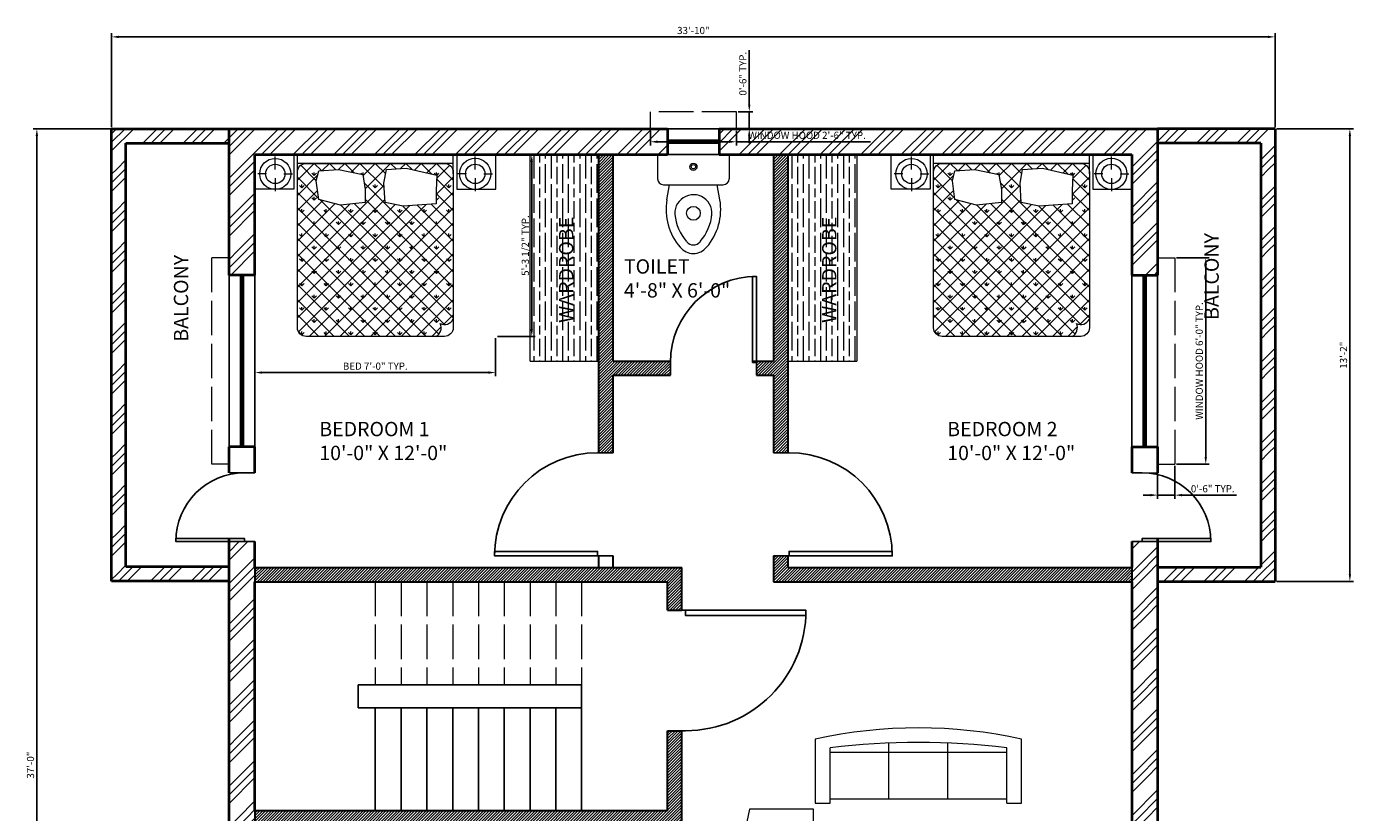
# Model space of a CAD drawing. Units: inches. Extents: x 2443635 to 2446153, y 1826255 to 1827341.
# Tile 10 of 16: x 2444253 to 2444716, y 1827067 to 1827341. Entities that reach past the tile are written whole.
import ezdxf

# ---------------------------------------------------------------- set-up
doc = ezdxf.new("R2010")
doc.units = ezdxf.units.IN
doc.linetypes.add('ACAD_ISO02W100', pattern=[15, 12, -3])
for name, color, linetype, lineweight in [('A-DIMS', 1, 'Continuous', 18), ('A-DOOR', 2, 'Continuous', 25), ('A-DOOR-HIDN', 2, 'ACAD_ISO02W100', 18), ('A-FLOR-CASE', 8, 'Continuous', 18), ('A-FLOR-CASE-PATT', 252, 'Continuous', 13), ('A-FLOR-FIXT', 9, 'Continuous', 18), ('A-FURN', 6, 'Continuous', 18), ('A-ROOM', 4, 'Continuous', 18), ('A-STAIR', 7, 'Continuous', 25), ('A-STAIR-OVHD', 7, 'ACAD_ISO02W100', 18), ('A-WALL-EXT', 7, 'Continuous', 40), ('A-WALL-INT', 9, 'Continuous', 30), ('A-WALL-OVHD', 7, 'ACAD_ISO02W100', 18), ('A-WALL-PATT', 8, 'Continuous', 13), ('A-WINDOW', 4, 'Continuous', 25)]:
    doc.layers.add(name, color=color, linetype=linetype, lineweight=lineweight)
doc.styles.get("Standard").update_dxf_attribs({"font": 'arial.ttf'})
doc.dimstyles.new('ISO-25', dxfattribs={"dimtxt": 2.5, "dimasz": 2.5, "dimexe": 1.25, "dimexo": 0.625, "dimtad": 1, "dimlunit": 4, "dimtxsty": 'Standard', "dimcen": 2.5, "dimadec": 0, "dimazin": 0, "dimtfac": 1, "dimtmove": 0, "dimatfit": 3, "dimfxl": 1, "dimarcsym": 0})

# ---------------------------------------------------------------- blocks, each defined once
blk = doc.blocks.new('*X6')
at = {"color": 0}
for p, q in [((0, 0), (0, 0)), ((-707, -141), (-734, -115)), ((-707, -141), (-707, -104)), ((-707, -141), (-681, -115)), ((-566, 0), (-566, 0)), ((-566, 0), (-566, 0)), ((-283, 0), (-283, 0)), ((-283, 0), (-283, 0)), ((-156, -126), (-168, -115)), ((-141, -141), (-142, -140)), ((-141, -141), (-141, -104)), ((-141, -141), (-115, -115)), ((120, -120), (115, -115)), ((283, 0), (283, 0)), ((566, 0), (566, 0)), ((699, -134), (681, -115)), ((707, -135), (707, -104)), ((710, -139), (734, -115)), ((-849, -283), (-875, -256)), ((-849, -283), (-849, -245)), ((-849, -283), (-822, -256)), ((0, -283), (-27, -256)), ((0, -283), (0, -245)), ((0, -283), (27, -256)), ((849, -283), (822, -256)), ((849, -283), (849, -245)), ((849, -283), (875, -256)), ((-707, -424), (-734, -398)), ((-707, -424), (-707, -387)), ((-707, -424), (-681, -398)), ((-116, -399), (-115, -398)), ((707, -424), (703, -420)), ((707, -424), (707, -387)), ((707, -424), (734, -398)), ((-849, -566), (-875, -539)), ((-849, -566), (-849, -528)), ((-849, -566), (-822, -539)), ((-566, -566), (-592, -539)), ((-566, -566), (-566, -528)), ((-566, -566), (-539, -539)), ((-283, -566), (-309, -539)), ((-283, -566), (-283, -528)), ((-283, -566), (-256, -539)), ((0, -566), (-27, -539)), ((0, -566), (0, -528)), ((0, -566), (27, -539)), ((283, -566), (256, -539)), ((283, -566), (283, -528)), ((283, -566), (309, -539)), ((566, -566), (539, -539)), ((566, -566), (566, -528)), ((566, -566), (592, -539)), ((849, -566), (822, -539)), ((849, -566), (849, -528)), ((849, -566), (875, -539)), ((-707, -707), (-734, -681)), ((-707, -707), (-707, -670)), ((-707, -707), (-681, -681)), ((-424, -707), (-451, -681)), ((-424, -707), (-424, -670)), ((-424, -707), (-398, -681)), ((-141, -707), (-168, -681)), ((-141, -707), (-141, -670)), ((-141, -707), (-115, -681)), ((141, -707), (115, -681)), ((141, -707), (141, -670)), ((141, -707), (168, -681)), ((424, -707), (398, -681)), ((424, -707), (424, -670)), ((424, -707), (451, -681)), ((707, -707), (681, -681)), ((707, -707), (707, -670)), ((707, -707), (734, -681)), ((-849, -849), (-875, -822)), ((-849, -849), (-849, -811)), ((-849, -849), (-822, -822)), ((-566, -849), (-592, -822)), ((-566, -849), (-566, -811)), ((-566, -849), (-539, -822)), ((-283, -849), (-309, -822)), ((-283, -849), (-283, -811)), ((-283, -849), (-256, -822)), ((0, -849), (-27, -822)), ((0, -849), (0, -811)), ((0, -849), (27, -822)), ((283, -849), (256, -822)), ((283, -849), (283, -811)), ((283, -849), (309, -822)), ((566, -849), (539, -822)), ((566, -849), (566, -811)), ((566, -849), (592, -822)), ((849, -849), (822, -822)), ((849, -849), (849, -811)), ((849, -849), (875, -822)), ((-707, -990), (-734, -963)), ((-707, -990), (-707, -952)), ((-707, -990), (-681, -963)), ((-424, -990), (-451, -963)), ((-424, -990), (-424, -952)), ((-424, -990), (-398, -963)), ((-141, -990), (-168, -963)), ((-141, -990), (-141, -952)), ((-141, -990), (-115, -963)), ((141, -990), (115, -963)), ((141, -990), (141, -952)), ((141, -990), (168, -963)), ((424, -990), (398, -963)), ((424, -990), (424, -952)), ((424, -990), (451, -963)), ((707, -990), (681, -963)), ((707, -990), (707, -952)), ((707, -990), (734, -963)), ((-849, -1131), (-875, -1105)), ((-849, -1131), (-849, -1094)), ((-849, -1131), (-822, -1105)), ((-566, -1131), (-592, -1105)), ((-566, -1131), (-566, -1094)), ((-566, -1131), (-539, -1105)), ((-283, -1131), (-309, -1105)), ((-283, -1131), (-283, -1094)), ((-283, -1131), (-256, -1105)), ((0, -1131), (-27, -1105)), ((0, -1131), (0, -1094)), ((0, -1131), (27, -1105)), ((283, -1131), (256, -1105)), ((283, -1131), (283, -1094)), ((283, -1131), (309, -1105)), ((566, -1131), (539, -1105)), ((566, -1131), (566, -1094)), ((566, -1131), (592, -1105)), ((849, -1131), (822, -1105)), ((849, -1131), (849, -1094)), ((849, -1131), (875, -1105)), ((-849, -1414), (-849, -1377)), ((-707, -1273), (-734, -1246)), ((-707, -1273), (-707, -1235)), ((-707, -1273), (-681, -1246)), ((-566, -1414), (-566, -1377)), ((-424, -1273), (-451, -1246)), ((-424, -1273), (-424, -1235)), ((-424, -1273), (-398, -1246)), ((-283, -1414), (-283, -1377)), ((-141, -1273), (-168, -1246)), ((-141, -1273), (-141, -1235)), ((-141, -1273), (-115, -1246)), ((0, -1414), (0, -1377)), ((141, -1273), (115, -1246)), ((141, -1273), (141, -1235)), ((141, -1273), (168, -1246)), ((283, -1414), (283, -1377)), ((424, -1273), (398, -1246)), ((424, -1273), (424, -1235)), ((424, -1273), (451, -1246)), ((566, -1414), (566, -1377)), ((707, -1273), (681, -1246)), ((707, -1273), (707, -1235)), ((707, -1273), (734, -1246)), ((849, -1414), (849, -1377)), ((-849, -1414), (-875, -1388)), ((-849, -1414), (-822, -1388)), ((-707, -1556), (-734, -1529)), ((-707, -1556), (-707, -1518)), ((-707, -1556), (-681, -1529)), ((-566, -1414), (-592, -1388)), ((-566, -1414), (-539, -1388)), ((-424, -1556), (-451, -1529)), ((-424, -1556), (-424, -1518)), ((-424, -1556), (-398, -1529)), ((-283, -1414), (-309, -1388)), ((-283, -1414), (-256, -1388)), ((-141, -1556), (-168, -1529)), ((-141, -1556), (-141, -1518)), ((-141, -1556), (-115, -1529)), ((0, -1414), (-27, -1388)), ((0, -1414), (27, -1388)), ((141, -1556), (115, -1529)), ((141, -1556), (141, -1518)), ((141, -1556), (168, -1529)), ((283, -1414), (256, -1388)), ((283, -1414), (309, -1388)), ((424, -1556), (398, -1529)), ((424, -1556), (424, -1518)), ((424, -1556), (451, -1529)), ((566, -1414), (539, -1388)), ((566, -1414), (592, -1388)), ((707, -1556), (681, -1529)), ((707, -1556), (707, -1518)), ((707, -1556), (734, -1529)), ((849, -1414), (822, -1388)), ((849, -1414), (875, -1388)), ((-849, -1697), (-875, -1671)), ((-849, -1697), (-849, -1660)), ((-849, -1697), (-822, -1671)), ((-566, -1697), (-592, -1671)), ((-566, -1697), (-566, -1660)), ((-566, -1697), (-539, -1671)), ((-283, -1697), (-309, -1671)), ((-283, -1697), (-283, -1660)), ((-283, -1697), (-256, -1671)), ((0, -1697), (-27, -1671)), ((0, -1697), (0, -1660)), ((0, -1697), (27, -1671)), ((283, -1697), (256, -1671)), ((283, -1697), (283, -1660)), ((283, -1697), (309, -1671)), ((566, -1697), (539, -1671)), ((566, -1697), (566, -1660)), ((566, -1697), (592, -1671)), ((849, -1697), (822, -1671)), ((849, -1697), (849, -1660)), ((849, -1697), (875, -1671)), ((-707, -1838), (-734, -1812)), ((-707, -1838), (-707, -1801)), ((-707, -1838), (-681, -1812)), ((-424, -1838), (-451, -1812)), ((-424, -1838), (-424, -1801)), ((-424, -1838), (-398, -1812)), ((-141, -1838), (-168, -1812)), ((-141, -1838), (-141, -1801)), ((-141, -1838), (-115, -1812)), ((141, -1838), (115, -1812)), ((141, -1838), (141, -1801)), ((141, -1838), (168, -1812)), ((424, -1838), (398, -1812)), ((424, -1838), (424, -1801)), ((424, -1838), (451, -1812)), ((707, -1838), (681, -1812)), ((707, -1838), (707, -1801)), ((707, -1838), (734, -1812)), ((-849, -1980), (-875, -1953)), ((-849, -1980), (-849, -1942)), ((-849, -1980), (-822, -1953)), ((-566, -1980), (-592, -1953)), ((-566, -1980), (-566, -1942)), ((-566, -1980), (-539, -1953)), ((-283, -1980), (-309, -1953)), ((-283, -1980), (-283, -1942)), ((-283, -1980), (-256, -1953)), ((0, -1980), (-27, -1953)), ((0, -1980), (0, -1942)), ((0, -1980), (27, -1953)), ((283, -1980), (256, -1953)), ((283, -1980), (283, -1942)), ((283, -1980), (309, -1953)), ((566, -1980), (539, -1953)), ((566, -1980), (566, -1942)), ((566, -1980), (592, -1953))]:
    blk.add_line(p, q, dxfattribs=at)
blk = doc.blocks.new('*X5')
at = {"color": 0}
for p, q in [((-900, -193), (-707, 0)), ((-623, -84), (-707, 0)), ((-614, -83), (-530, 0)), ((-457, -74), (-530, 0)), ((-425, -72), (-354, 0)), ((-245, -108), (-354, 0)), ((-278, -101), (-177, 0)), ((103, -280), (-177, 0)), ((-142, -142), (0, 0)), ((-117, -294), (177, 0)), ((120, -120), (0, 0)), ((241, -64), (177, 0)), ((292, -61), (354, 0)), ((426, -72), (354, 0)), ((452, -78), (530, 0)), ((654, -123), (530, 0)), ((596, -111), (707, 0)), ((900, -193), (707, 0)), ((-900, -370), (-667, -137)), ((-683, -201), (-862, -22)), ((708, -175), (862, -22)), ((-656, -405), (-900, -161)), ((-900, -1254), (101, -252)), ((900, -1254), (-128, -225)), ((703, -358), (900, -161)), ((900, -370), (708, -178)), ((-900, -546), (-668, -314)), ((735, -1973), (-900, -337)), ((-900, -1430), (112, -418)), ((-900, -723), (-605, -429)), ((-763, -2000), (900, -337)), ((801, -1862), (-641, -419)), ((900, -1430), (-116, -415)), ((900, -546), (703, -349)), ((-900, -900), (-465, -465)), ((-900, -1077), (-293, -470)), ((-900, -1607), (231, -476)), ((-900, -1784), (394, -489)), ((586, -2000), (-900, -514)), ((-888, -1948), (586, -475)), ((-586, -2000), (900, -514)), ((900, -1784), (-404, -480)), ((900, -1607), (-243, -465)), ((900, -1077), (317, -494)), ((900, -900), (483, -483)), ((900, -723), (647, -470)), ((409, -2000), (-900, -691)), ((-409, -2000), (900, -691)), ((232, -2000), (-900, -868)), ((-232, -2000), (900, -868)), ((55, -2000), (-900, -1045)), ((-55, -2000), (900, -1045)), ((-121, -2000), (-900, -1221)), ((121, -2000), (900, -1221)), ((-298, -2000), (-900, -1398)), ((298, -2000), (900, -1398)), ((-475, -2000), (-900, -1575)), ((475, -2000), (900, -1575)), ((-652, -2000), (-900, -1752)), ((790, -1861), (900, -1752)), ((-835, -1994), (-894, -1935)), ((652, -2000), (761, -1890))]:
    blk.add_line(p, q, dxfattribs=at)
blk = doc.blocks.new('A$C190D2546')
at = {"layer": 'A-FURN'}
for p, q in [((285, 1928), (285, 2078)), ((541, 2100), (2341, 2100)), ((541, 1881), (541, 2100)), ((2341, 2000), (541, 2000)), ((2341, 1881), (2341, 2100)), ((2596, 1929), (2596, 2079)), ((185, 1878), (85, 1878)), ((385, 1878), (485, 1878)), ((2496, 1879), (2396, 1879)), ((2696, 1879), (2796, 1879)), ((285, 1828), (285, 1678)), ((2596, 1829), (2596, 1679))]:
    blk.add_line(p, q, dxfattribs=at)
for points in [[(500, 2101), (500, 1701), (50, 1701), (50, 2101)], [(2382, 2101), (2382, 1701), (2832, 1701), (2832, 2101)], [(787, 1584), (758, 1799), (787, 1914), (1016, 1928), (1296, 1871), (1325, 1699), (1325, 1548), (1038, 1519)], [(1555, 1548), (1541, 1771), (1569, 1928), (1799, 1943), (2151, 1864), (2144, 1685), (2144, 1534), (1763, 1505)]]:
    blk.add_lwpolyline(points, close=True, dxfattribs=at)
blk.add_lwpolyline([(641, 2000), (2241, 2000, -0.414214), (2341, 1900), (2341, 100, -0.414214), (2241, 0), (641, 0, -0.414214), (541, 100), (541, 1900, -0.414214)], format="xyb", close=True, dxfattribs=at)
for centre, radius in [((285, 1878), 180), ((2596, 1879), 180), ((285, 1878), 112), ((2596, 1879), 112)]:
    blk.add_circle(centre, radius, dxfattribs=at)
for centre, start, end in [((2241, 250), 243.4349, 333.4349), ((2091, 100), 296.5651, 26.5651)]:
    blk.add_arc(centre, 112, start, end, dxfattribs=at)
for name in ['*X5', '*X6']:
    blk.add_blockref(name, (1441, 2000), dxfattribs=at)
blk = doc.blocks.new('*U2')
for p, q in [((0, 0), (0, -6)), ((40, 0), (40, -6))]:
    blk.add_line(p, q)
blk.add_lwpolyline([(0, 0), (0, 40), (1.75, 40), (1.75, 0)], close=True)
blk.add_arc((0, 0), 40, 0, 90)
blk = doc.blocks.new('*U3')
for p, q in [((0, 0), (0, -6)), ((-40, 0), (-40, -6))]:
    blk.add_line(p, q)
blk.add_lwpolyline([(0, 0), (0, 40), (-1.75, 40), (-1.75, 0)], close=True)
blk.add_arc((0, 0), 40, 90, 180)
blk = doc.blocks.new('*U14')
for p, q in [((0, 0), (0, -6)), ((40, 0), (40, -6))]:
    blk.add_line(p, q)
blk.add_lwpolyline([(0, 0), (0, 40), (1.75, 40), (1.75, 0)], close=True)
blk.add_arc((0, 0), 40, 0, 90)
blk = doc.blocks.new('SOFA-3-SEAT')
at = {"transparency": 33554687}
for p, q in [((0, 22.29), (0, 0)), ((5.14, 0), (5.14, 19.31)), ((25.71, 1.34), (25.71, 20.94)), ((46.29, 1.34), (46.29, 20.94)), ((66.86, 0), (66.86, 19.31)), ((72, 0), (72, 22.29)), ((66.86, 17.67), (5.14, 17.67)), ((0, 0), (5.14, 0)), ((66.86, 1.34), (5.14, 1.34)), ((66.86, 0), (72, 0))]:
    blk.add_line(p, q, dxfattribs=at)
for centre, radius, start, end in [((36, -137.71), 164, 77.3196, 102.6804), ((36, -239.71), 260.86, 83.2065, 96.7935)]:
    blk.add_arc(centre, radius, start, end, dxfattribs=at)
blk = doc.blocks.new('WIN-18-PLAN')
at = {"transparency": 33554687}
for p, q in [((18, 9), (0, 9)), ((0, 9), (0, 0)), ((0, 5), (18, 5)), ((0.5, 5), (0.5, 4)), ((17.5, 4), (17.5, 5)), ((18, 0), (18, 9)), ((0, 4), (18, 4)), ((0.5, 4.5), (18, 4.5)), ((0, 0), (18, 0))]:
    blk.add_line(p, q, dxfattribs=at)
blk = doc.blocks.new('WIN-60-PLAN')
at = {"transparency": 33554687}
for p, q in [((0, 0), (0, 60)), ((0, 60), (9, 60)), ((4, 60), (4, 0)), ((4, 59.5), (5, 59.5)), ((4.5, 59.5), (4.5, 0.5)), ((5, 60), (5, 0)), ((9, 60), (9, 0)), ((5, 0.5), (4, 0.5)), ((9, 0), (0, 0))]:
    blk.add_line(p, q, dxfattribs=at)
blk = doc.blocks.new('WIN-60-STRIP-PLAN')
at = {"transparency": 33554687}
for p, q in [((0, 0), (0, 60)), ((4, 60), (4, 0)), ((4.5, 59.5), (4.5, 0.5)), ((5, 60), (5, 0)), ((9, 60), (9, 0))]:
    blk.add_line(p, q, dxfattribs=at)
blk = doc.blocks.new('WINDOW-HOOD-72-PLAN')
at = {"transparency": 33554687}
for p, q in [((0, 72), (6, 72)), ((6, 72), (6, 0)), ((0, 0), (6, 0))]:
    blk.add_line(p, q, dxfattribs=at)
blk = doc.blocks.new('WINDOW-HOOD-30-PLAN')
at = {"transparency": 33554687}
for p, q in [((30, 6), (0, 6)), ((0, 0), (0, 6)), ((30, 0), (30, 6))]:
    blk.add_line(p, q, dxfattribs=at)
blk = doc.blocks.new('*D52')
at = {"layer": 'A-DIMS', "color": 0, "lineweight": -2, "transparency": 16777216}
for p, q in [((2444332.55, 1827232.23), (2444332.55, 1827219)), ((2444416.55, 1827232.23), (2444416.55, 1827219)), ((2444335.05, 1827220.25), (2444414.05, 1827220.25))]:
    blk.add_line(p, q, dxfattribs=at)
at = {"layer": 'A-DIMS', "color": 0, "transparency": 16777216}
for points in [[(2444335.05, 1827220.67), (2444335.05, 1827219.84), (2444332.55, 1827220.25)], [(2444414.05, 1827220.67), (2444414.05, 1827219.84), (2444416.55, 1827220.25)]]:
    blk.add_solid(points, dxfattribs=at)
at = {"layer": 'Defpoints', "color": 0, "transparency": 16777216}
for p in [(2444332.55, 1827232.85), (2444416.55, 1827232.85), (2444416.55, 1827220.25)]:
    blk.add_point(p, dxfattribs=at)
at = {"layer": 'A-DIMS', "color": 0, "transparency": 16777216, "insert": (2444374.55, 1827222.16), "char_height": 2.5, "attachment_point": 5}
blk.add_mtext('BED 7\'-0" TYP.', dxfattribs=at)
blk = doc.blocks.new('*D53')
at = {"layer": 'A-DIMS', "color": 0, "lineweight": -2, "transparency": 16777216}
for p, q in [((2444417.18, 1827296.29), (2444430.4, 1827296.29)), ((2444429.15, 1827235.35), (2444429.15, 1827293.79)), ((2444417.18, 1827232.85), (2444430.4, 1827232.85))]:
    blk.add_line(p, q, dxfattribs=at)
at = {"layer": 'A-DIMS', "color": 0, "transparency": 16777216}
for points in [[(2444428.74, 1827293.79), (2444429.57, 1827293.79), (2444429.15, 1827296.29)], [(2444428.74, 1827235.35), (2444429.57, 1827235.35), (2444429.15, 1827232.85)]]:
    blk.add_solid(points, dxfattribs=at)
at = {"layer": 'Defpoints', "color": 0, "transparency": 16777216}
for p in [(2444416.55, 1827296.29), (2444429.15, 1827296.29), (2444416.55, 1827232.85)]:
    blk.add_point(p, dxfattribs=at)
at = {"layer": 'A-DIMS', "color": 0, "transparency": 16777216, "insert": (2444427.23, 1827264.57), "char_height": 2.5, "attachment_point": 5, "rotation": 90}
blk.add_mtext('5\'-3 1/2" TYP.', dxfattribs=at)
blk = doc.blocks.new('*D58')
at = {"layer": 'A-DIMS', "color": 0, "lineweight": -2, "transparency": 16777216}
for p, q in [((2444654.18, 1827260.29), (2444665.6, 1827260.29)), ((2444664.35, 1827190.79), (2444664.35, 1827257.79)), ((2444654.18, 1827188.29), (2444665.6, 1827188.29))]:
    blk.add_line(p, q, dxfattribs=at)
at = {"layer": 'A-DIMS', "color": 0, "transparency": 16777216}
for points in [[(2444663.94, 1827257.79), (2444664.77, 1827257.79), (2444664.35, 1827260.29)], [(2444663.94, 1827190.79), (2444664.77, 1827190.79), (2444664.35, 1827188.29)]]:
    blk.add_solid(points, dxfattribs=at)
at = {"layer": 'Defpoints', "color": 0, "transparency": 16777216}
for p in [(2444653.55, 1827260.29), (2444664.35, 1827260.29), (2444653.55, 1827188.29)]:
    blk.add_point(p, dxfattribs=at)
at = {"layer": 'A-DIMS', "color": 0, "transparency": 16777216, "insert": (2444662.43, 1827224.29), "char_height": 2.5, "attachment_point": 5, "rotation": 90}
blk.add_mtext('WINDOW HOOD 6\'-0" TYP.', dxfattribs=at)
blk = doc.blocks.new('*D59')
at = {"layer": 'A-DIMS', "color": 0, "lineweight": -2, "transparency": 16777216}
for p, q in [((2444647.55, 1827187.66), (2444647.55, 1827176.24)), ((2444653.55, 1827187.66), (2444653.55, 1827176.24)), ((2444645.05, 1827177.49), (2444642.55, 1827177.49)), ((2444647.55, 1827177.49), (2444653.55, 1827177.49)), ((2444656.05, 1827177.49), (2444675.04, 1827177.49))]:
    blk.add_line(p, q, dxfattribs=at)
at = {"layer": 'A-DIMS', "color": 0, "transparency": 16777216}
for points in [[(2444645.05, 1827177.9), (2444645.05, 1827177.07), (2444647.55, 1827177.49)], [(2444656.05, 1827177.9), (2444656.05, 1827177.07), (2444653.55, 1827177.49)]]:
    blk.add_solid(points, dxfattribs=at)
at = {"layer": 'Defpoints', "color": 0, "transparency": 16777216}
for p in [(2444647.55, 1827188.29), (2444653.55, 1827188.29), (2444653.55, 1827177.49)]:
    blk.add_point(p, dxfattribs=at)
at = {"layer": 'A-DIMS', "color": 0, "transparency": 16777216, "insert": (2444666.8, 1827179.39), "char_height": 2.5, "attachment_point": 5}
blk.add_mtext('0\'-6" TYP.', dxfattribs=at)
blk = doc.blocks.new('*D86')
at = {"layer": 'A-DIMS', "color": 0, "lineweight": -2, "transparency": 16777216}
for p, q in [((2444470.55, 1827304.66), (2444470.55, 1827299.54)), ((2444500.55, 1827304.66), (2444500.55, 1827299.54)), ((2444473.05, 1827300.79), (2444498.05, 1827300.79)), ((2444500.55, 1827300.79), (2444547.39, 1827300.79))]:
    blk.add_line(p, q, dxfattribs=at)
at = {"layer": 'A-DIMS', "color": 0, "transparency": 16777216}
for points in [[(2444473.05, 1827301.2), (2444473.05, 1827300.37), (2444470.55, 1827300.79)], [(2444498.05, 1827301.2), (2444498.05, 1827300.37), (2444500.55, 1827300.79)]]:
    blk.add_solid(points, dxfattribs=at)
at = {"layer": 'Defpoints', "color": 0, "transparency": 16777216}
for p in [(2444470.55, 1827305.29), (2444500.55, 1827305.29), (2444500.55, 1827300.79)]:
    blk.add_point(p, dxfattribs=at)
at = {"layer": 'A-DIMS', "color": 0, "transparency": 16777216, "insert": (2444525.22, 1827302.71), "char_height": 2.5, "attachment_point": 5}
blk.add_mtext('WINDOW HOOD 2\'-6" TYP.', dxfattribs=at)
blk = doc.blocks.new('*D87')
at = {"layer": 'A-DIMS', "color": 0, "lineweight": -2, "transparency": 16777216}
for p, q in [((2444505.05, 1827313.79), (2444505.05, 1827332.78)), ((2444501.18, 1827311.29), (2444506.3, 1827311.29)), ((2444505.05, 1827305.29), (2444505.05, 1827311.29)), ((2444501.18, 1827305.29), (2444506.3, 1827305.29)), ((2444505.05, 1827302.79), (2444505.05, 1827300.29))]:
    blk.add_line(p, q, dxfattribs=at)
at = {"layer": 'A-DIMS', "color": 0, "transparency": 16777216}
for points in [[(2444504.64, 1827313.79), (2444505.47, 1827313.79), (2444505.05, 1827311.29)], [(2444504.64, 1827302.79), (2444505.47, 1827302.79), (2444505.05, 1827305.29)]]:
    blk.add_solid(points, dxfattribs=at)
at = {"layer": 'Defpoints', "color": 0, "transparency": 16777216}
for p in [(2444500.55, 1827311.29), (2444505.05, 1827311.29), (2444500.55, 1827305.29)]:
    blk.add_point(p, dxfattribs=at)
at = {"layer": 'A-DIMS', "color": 0, "transparency": 16777216, "insert": (2444503.15, 1827324.53), "char_height": 2.5, "attachment_point": 5, "rotation": 90}
blk.add_mtext('0\'-6" TYP.', dxfattribs=at)
blk = doc.blocks.new('*D94')
at = {"layer": 'A-DIMS', "color": 0, "lineweight": -2, "transparency": 16777216}
for p, q in [((2444282.55, 1827305.91), (2444282.55, 1827338.64)), ((2444285.05, 1827337.39), (2444686.05, 1827337.39)), ((2444688.55, 1827305.91), (2444688.55, 1827338.64))]:
    blk.add_line(p, q, dxfattribs=at)
at = {"layer": 'A-DIMS', "color": 0, "transparency": 16777216}
for points in [[(2444285.05, 1827337.8), (2444285.05, 1827336.97), (2444282.55, 1827337.39)], [(2444686.05, 1827337.8), (2444686.05, 1827336.97), (2444688.55, 1827337.39)]]:
    blk.add_solid(points, dxfattribs=at)
at = {"layer": 'Defpoints', "color": 0, "transparency": 16777216}
for p in [(2444688.55, 1827337.39), (2444282.55, 1827305.29), (2444688.55, 1827305.29)]:
    blk.add_point(p, dxfattribs=at)
at = {"layer": 'A-DIMS', "color": 0, "transparency": 16777216, "insert": (2444485.55, 1827339.29), "char_height": 2.5, "attachment_point": 5}
blk.add_mtext('33\'-10"', dxfattribs=at)
blk = doc.blocks.new('*D95')
at = {"layer": 'A-DIMS', "color": 0, "lineweight": -2, "transparency": 16777216}
for p, q in [((2444322.93, 1827305.29), (2444255.2, 1827305.29)), ((2444256.45, 1826863.79), (2444256.45, 1827302.79)), ((2444322.93, 1826861.29), (2444255.2, 1826861.29))]:
    blk.add_line(p, q, dxfattribs=at)
at = {"layer": 'A-DIMS', "color": 0, "transparency": 16777216}
for points in [[(2444256.04, 1827302.79), (2444256.87, 1827302.79), (2444256.45, 1827305.29)], [(2444256.04, 1826863.79), (2444256.87, 1826863.79), (2444256.45, 1826861.29)]]:
    blk.add_solid(points, dxfattribs=at)
at = {"layer": 'Defpoints', "color": 0, "transparency": 16777216}
for p in [(2444256.45, 1827305.29), (2444323.55, 1827305.29), (2444323.55, 1826861.29)]:
    blk.add_point(p, dxfattribs=at)
at = {"layer": 'A-DIMS', "color": 0, "transparency": 16777216, "insert": (2444254.55, 1827083.29), "char_height": 2.5, "attachment_point": 5, "rotation": 90}
blk.add_mtext('37\'-0"', dxfattribs=at)
blk = doc.blocks.new('*D96')
at = {"layer": 'A-DIMS', "color": 0, "lineweight": -2, "transparency": 16777216}
for p, q in [((2444689.18, 1827305.29), (2444715.9, 1827305.29)), ((2444714.65, 1827149.86), (2444714.65, 1827302.79)), ((2444689.18, 1827147.36), (2444715.9, 1827147.36))]:
    blk.add_line(p, q, dxfattribs=at)
at = {"layer": 'A-DIMS', "color": 0, "transparency": 16777216}
for points in [[(2444714.24, 1827302.79), (2444715.07, 1827302.79), (2444714.65, 1827305.29)], [(2444714.24, 1827149.86), (2444715.07, 1827149.86), (2444714.65, 1827147.36)]]:
    blk.add_solid(points, dxfattribs=at)
at = {"layer": 'Defpoints', "color": 0, "transparency": 16777216}
for p in [(2444688.55, 1827305.29), (2444714.65, 1827305.29), (2444688.55, 1827147.36)]:
    blk.add_point(p, dxfattribs=at)
at = {"layer": 'A-DIMS', "color": 0, "transparency": 16777216, "insert": (2444712.75, 1827226.32), "char_height": 2.5, "attachment_point": 5, "rotation": 90}
blk.add_mtext('13\'-2"', dxfattribs=at)

msp = doc.modelspace()

# ---------------------------------------------------------------- hatches: boundary and pattern name
at = {"layer": 'A-FLOR-CASE-PATT'}
h = msp.add_hatch(dxfattribs=at)
h.set_pattern_fill('GOST_WOOD', color=256)
h.paths.add_polyline_path([(2444452.553, 1827296.288), (2444428.553, 1827296.288), (2444428.553, 1827224.288), (2444452.553, 1827224.288)])
h.paths.add_polyline_path([(2444542.553, 1827296.288), (2444518.553, 1827296.288), (2444518.553, 1827224.288), (2444542.553, 1827224.288)])
at = {"layer": 'A-WALL-PATT'}
h = msp.add_hatch(dxfattribs=at)
h.set_pattern_fill('GOST_GROUND', color=256)
h.paths.add_polyline_path([(2444332.553, 1827147.288), (2444332.553, 1827152.288), (2444332.553, 1827161.288), (2444328.953, 1827161.288), (2444323.553, 1827161.288), (2444323.553, 1826984.288), (2444332.553, 1826984.288), (2444332.553, 1827062.288), (2444332.553, 1827067.288)])
h.paths.add_polyline_path([(2444332.553, 1826948.288), (2444323.553, 1826948.288), (2444323.553, 1826861.288), (2444374.553, 1826861.288), (2444374.553, 1826870.288), (2444332.553, 1826870.288)])
h.paths.add_polyline_path([(2444647.553, 1826941.288), (2444638.553, 1826941.288), (2444638.553, 1826935.288), (2444638.553, 1826930.288), (2444638.553, 1826870.288), (2444457.553, 1826870.288), (2444452.553, 1826870.288), (2444410.553, 1826870.288), (2444410.553, 1826861.288), (2444647.553, 1826861.288)])
h.paths.add_polyline_path([(2444647.553, 1827161.288), (2444638.553, 1827161.288), (2444638.553, 1827152.288), (2444638.553, 1827147.288), (2444638.553, 1826989.288), (2444647.553, 1826989.288)])
h.paths.add_polyline_path([(2444647.553, 1827305.288), (2444494.553, 1827305.288), (2444494.553, 1827296.288), (2444498.051, 1827296.288), (2444638.553, 1827296.288), (2444638.553, 1827254.288), (2444647.553, 1827254.288)])
h.paths.add_polyline_path([(2444476.553, 1827305.288), (2444323.553, 1827305.288), (2444323.553, 1827254.288), (2444332.553, 1827254.288), (2444332.553, 1827296.288), (2444346.141, 1827296.288), (2444476.553, 1827296.288)])
h.paths.add_polyline_path([(2444323.553, 1827305.288), (2444282.553, 1827305.288), (2444282.553, 1827147.459), (2444323.553, 1827147.459), (2444323.553, 1827152.459), (2444287.553, 1827152.459), (2444287.553, 1827300.288), (2444323.553, 1827300.288)])
h.paths.add_polyline_path([(2444688.553, 1827305.288), (2444647.553, 1827305.288), (2444647.553, 1827300.288), (2444683.553, 1827300.288), (2444683.553, 1827152.362), (2444647.553, 1827152.362), (2444647.553, 1827147.362), (2444688.553, 1827147.362)])
h = msp.add_hatch(dxfattribs=at)
h.set_pattern_fill('JIS_WOOD', color=256)
h.paths.add_polyline_path([(2444481.553, 1827095.288), (2444476.553, 1827095.288), (2444476.553, 1827067.288), (2444332.553, 1827067.288), (2444332.553, 1827062.288), (2444481.553, 1827062.288)])
h.paths.add_polyline_path([(2444457.553, 1827020.288), (2444452.553, 1827020.288), (2444452.553, 1826870.288), (2444457.553, 1826870.288), (2444457.553, 1826930.288), (2444530.053, 1826930.288), (2444530.053, 1826935.288), (2444457.553, 1826935.288)])
h.paths.add_polyline_path([(2444457.553, 1827062.288), (2444452.553, 1827062.288), (2444452.553, 1827056.288), (2444457.553, 1827056.288)])
h.paths.add_polyline_path([(2444638.553, 1826935.288), (2444566.053, 1826935.288), (2444566.053, 1826930.288), (2444638.553, 1826930.288)])
h.paths.add_polyline_path([(2444638.553, 1827152.288), (2444518.553, 1827152.288), (2444518.553, 1827156.288), (2444513.553, 1827156.288), (2444513.553, 1827147.288), (2444638.553, 1827147.288)])
h.paths.add_polyline_path([(2444518.553, 1827296.288), (2444513.553, 1827296.288), (2444513.553, 1827224.288), (2444507.553, 1827224.288), (2444507.553, 1827223.788), (2444507.553, 1827219.288), (2444513.553, 1827219.288), (2444513.553, 1827192.288), (2444518.553, 1827192.288)])
h.paths.add_polyline_path([(2444477.553, 1827223.788, -0.0041669), (2444477.557, 1827224.288), (2444457.553, 1827224.288), (2444457.553, 1827296.288), (2444452.553, 1827296.288), (2444452.553, 1827192.288), (2444457.553, 1827192.288), (2444457.553, 1827219.288), (2444477.553, 1827219.288)])
h.paths.add_polyline_path([(2444481.553, 1827152.288), (2444332.553, 1827152.288), (2444332.553, 1827147.288), (2444476.553, 1827147.288), (2444476.553, 1827137.288), (2444481.553, 1827137.288)])

# ---------------------------------------------------------------- linework, layer by layer
at = {"layer": 'A-DOOR-HIDN'}
for p, q in [((2444332.553, 1827185.288), (2444323.553, 1827185.288)), ((2444638.553, 1827185.288), (2444647.553, 1827185.288)), ((2444332.553, 1827161.288), (2444323.553, 1827161.288)), ((2444638.553, 1827161.288), (2444647.553, 1827161.288))]:
    msp.add_line(p, q, dxfattribs=at)
at = {"layer": 'A-FLOR-CASE'}
for p, q in [((2444428.553, 1827224.288), (2444428.553, 1827296.288)), ((2444542.553, 1827296.288), (2444542.553, 1827224.288)), ((2444428.553, 1827224.288), (2444452.553, 1827224.288)), ((2444518.553, 1827224.288), (2444542.553, 1827224.288))]:
    msp.add_line(p, q, dxfattribs=at)
at = {"layer": 'A-FLOR-FIXT'}
for p, q in [((2444473.054, 1827296.288), (2444476.553, 1827296.288)), ((2444473.054, 1827296.288), (2444473.054, 1827287.865)), ((2444494.553, 1827296.288), (2444498.051, 1827296.288)), ((2444498.051, 1827296.288), (2444498.051, 1827287.865)), ((2444475.116, 1827285.803), (2444495.989, 1827285.803)), ((2444476.304, 1827280.555), (2444477.218, 1827285.795)), ((2444494.801, 1827280.555), (2444493.887, 1827285.795))]:
    msp.add_line(p, q, dxfattribs=at)
for centre, radius in [((2444485.553, 1827292.053), 1.25), ((2444485.553, 1827292.053), 0.75), ((2444485.558, 1827275.824), 2.41)]:
    msp.add_circle(centre, radius, dxfattribs=at)
for centre, radius, start, end in [((2444475.116, 1827287.865), 2.062, 180, 270), ((2444495.989, 1827287.865), 2.062, 270, 0), ((2444496.007, 1827277.119), 20, 170.10608, 221.06503), ((2444485.558, 1827275.824), 6.479, 347.37133, 190.68391), ((2444475.098, 1827277.119), 20, 318.93497, 9.89392), ((2444496.007, 1827277.119), 17, 185.68603, 221.06503), ((2444475.098, 1827277.119), 17, 318.93497, 355.06328), ((2444485.553, 1827267.803), 3, 219.57421, 270), ((2444485.553, 1827267.803), 3, 270, 320.42579), ((2444485.553, 1827267.803), 6, 219.57421, 270), ((2444485.553, 1827267.803), 6, 270, 320.42579)]:
    msp.add_arc(centre, radius, start, end, dxfattribs=at)
at = {"layer": 'A-STAIR'}
for p, q in [((2444368.553, 1827111.288), (2444446.553, 1827111.288)), ((2444368.553, 1827103.288), (2444368.553, 1827111.288)), ((2444446.553, 1827067.288), (2444446.553, 1827111.288)), ((2444446.553, 1827103.288), (2444368.553, 1827103.288)), ((2444374.553, 1827067.288), (2444374.553, 1827103.288)), ((2444383.553, 1827067.288), (2444383.553, 1827103.288)), ((2444392.553, 1827067.288), (2444392.553, 1827103.288)), ((2444401.553, 1827067.288), (2444401.553, 1827103.288)), ((2444410.553, 1827067.288), (2444410.553, 1827103.288)), ((2444419.553, 1827067.288), (2444419.553, 1827103.288)), ((2444428.553, 1827067.288), (2444428.553, 1827103.288)), ((2444437.553, 1827067.288), (2444437.553, 1827103.288))]:
    msp.add_line(p, q, dxfattribs=at)
at = {"layer": 'A-STAIR-OVHD'}
for p, q in [((2444374.553, 1827147.288), (2444374.553, 1827111.288)), ((2444383.553, 1827147.288), (2444383.553, 1827111.288)), ((2444392.553, 1827147.288), (2444392.553, 1827111.288)), ((2444401.553, 1827147.288), (2444401.553, 1827111.288)), ((2444410.553, 1827147.288), (2444410.553, 1827111.288)), ((2444419.553, 1827147.288), (2444419.553, 1827111.288)), ((2444428.553, 1827147.288), (2444428.553, 1827111.288)), ((2444437.553, 1827147.288), (2444437.553, 1827111.288)), ((2444446.553, 1827147.288), (2444446.553, 1827111.288))]:
    msp.add_line(p, q, dxfattribs=at)
at = {"layer": 'A-WALL-EXT'}
for p, q in [((2444282.553, 1827147.459), (2444282.553, 1827305.288)), ((2444282.553, 1827305.288), (2444323.553, 1827305.288)), ((2444323.553, 1827305.288), (2444476.553, 1827305.288)), ((2444323.553, 1827254.288), (2444323.553, 1827305.288)), ((2444476.553, 1827305.288), (2444476.553, 1827296.288)), ((2444494.553, 1827305.288), (2444647.553, 1827305.288)), ((2444494.553, 1827305.288), (2444494.553, 1827296.288)), ((2444647.553, 1827305.288), (2444647.553, 1827254.288)), ((2444688.553, 1827305.288), (2444647.553, 1827305.288)), ((2444688.553, 1827305.288), (2444688.553, 1827147.362)), ((2444287.553, 1827152.459), (2444287.553, 1827300.288)), ((2444287.553, 1827300.288), (2444323.553, 1827300.288)), ((2444683.553, 1827300.288), (2444647.553, 1827300.288)), ((2444683.553, 1827300.288), (2444683.553, 1827152.362)), ((2444332.553, 1827296.288), (2444476.553, 1827296.288)), ((2444332.553, 1827254.288), (2444332.553, 1827296.288)), ((2444494.553, 1827296.288), (2444638.553, 1827296.288)), ((2444638.553, 1827296.288), (2444638.553, 1827254.288)), ((2444332.553, 1827254.288), (2444323.553, 1827254.288)), ((2444638.553, 1827254.288), (2444647.553, 1827254.288)), ((2444332.553, 1827194.288), (2444323.553, 1827194.288)), ((2444323.553, 1827185.288), (2444323.553, 1827194.288)), ((2444332.553, 1827185.288), (2444332.553, 1827194.288)), ((2444638.553, 1827194.288), (2444647.553, 1827194.288)), ((2444638.553, 1827194.288), (2444638.553, 1827185.288)), ((2444647.553, 1827194.288), (2444647.553, 1827185.288)), ((2444323.553, 1826984.288), (2444323.553, 1827162.338)), ((2444332.553, 1827152.288), (2444332.553, 1827161.288)), ((2444638.553, 1827161.288), (2444638.553, 1827152.288)), ((2444647.553, 1827162.338), (2444647.553, 1826989.288)), ((2444323.553, 1827152.459), (2444287.553, 1827152.459)), ((2444647.553, 1827152.362), (2444683.553, 1827152.362)), ((2444323.553, 1827147.459), (2444282.553, 1827147.459)), ((2444332.553, 1827067.288), (2444332.553, 1827147.288)), ((2444638.553, 1827147.288), (2444638.553, 1826989.288)), ((2444647.553, 1827147.362), (2444688.553, 1827147.362))]:
    msp.add_line(p, q, dxfattribs=at)
at = {"layer": 'A-WALL-INT'}
for p, q in [((2444452.553, 1827192.288), (2444452.553, 1827296.288)), ((2444457.553, 1827224.288), (2444457.553, 1827296.288)), ((2444513.553, 1827296.288), (2444513.553, 1827224.288)), ((2444518.553, 1827296.288), (2444518.553, 1827192.288)), ((2444457.553, 1827224.288), (2444477.557, 1827224.288)), ((2444506.24, 1827224.288), (2444513.553, 1827224.288)), ((2444457.553, 1827219.288), (2444477.553, 1827219.288)), ((2444457.553, 1827192.288), (2444457.553, 1827219.288)), ((2444507.553, 1827219.288), (2444513.553, 1827219.288)), ((2444513.553, 1827219.288), (2444513.553, 1827192.288)), ((2444452.553, 1827152.288), (2444452.553, 1827156.288)), ((2444457.553, 1827152.288), (2444457.553, 1827156.288)), ((2444513.553, 1827156.288), (2444513.553, 1827147.288)), ((2444518.553, 1827156.288), (2444518.553, 1827152.288)), ((2444332.553, 1827152.288), (2444481.553, 1827152.288)), ((2444332.553, 1827152.288), (2444332.553, 1827147.288)), ((2444481.553, 1827137.288), (2444481.553, 1827152.288)), ((2444518.553, 1827152.288), (2444638.553, 1827152.288)), ((2444638.553, 1827152.288), (2444638.553, 1827147.288)), ((2444332.553, 1827147.288), (2444476.553, 1827147.288)), ((2444476.553, 1827137.288), (2444476.553, 1827147.288)), ((2444513.553, 1827147.288), (2444638.553, 1827147.288)), ((2444476.553, 1827137.288), (2444481.553, 1827137.288)), ((2444476.553, 1827067.288), (2444476.553, 1827095.288)), ((2444476.553, 1827095.288), (2444481.553, 1827095.288)), ((2444481.553, 1827062.288), (2444481.553, 1827095.288)), ((2444476.553, 1827067.288), (2444332.553, 1827067.288)), ((2444332.553, 1827067.288), (2444332.553, 1827062.288))]:
    msp.add_line(p, q, dxfattribs=at)
at = {"layer": 'A-WINDOW'}
for p, q in [((2444476.553, 1827305.288), (2444476.553, 1827296.288)), ((2444638.553, 1827254.288), (2444647.553, 1827254.288))]:
    msp.add_line(p, q, dxfattribs=at)

# ---------------------------------------------------------------- block references
at = {"layer": 'A-DOOR', "xscale": 0.75, "yscale": 0.75, "zscale": 0.75}
msp.add_blockref('*U3', (2444507.553, 1827223.788), dxfattribs=at)
at = {"layer": 'A-DOOR'}
for name, p, xscale, yscale, zscale, rotation in [('*U2', (2444452.153, 1827156.288), 0.9, 0.9, 0.9, 90), ('*U2', (2444518.953, 1827156.288), -0.9, 0.9, 0.9, 270), ('*U3', (2444328.953, 1827161.288), -0.6000000000000001, 0.6000000000000001, 0.6000000000000001, 90), ('*U3', (2444642.153, 1827161.288), 0.6000000000000001, 0.6000000000000001, 0.6000000000000001, 270), ('*U14', (2444482.853, 1827137.288), 1.05, 1.05, 1.05, 270)]:
    msp.add_blockref(name, p, dxfattribs=dict(at, xscale=xscale, yscale=yscale, zscale=zscale, rotation=rotation))
at = {"layer": 'A-FURN', "xscale": 0.0301964232523521, "yscale": 0.0301964232523521, "zscale": 0.0301964232523521}
for p in [(2444331.043, 1827232.854), (2444553.043, 1827232.854)]:
    msp.add_blockref('A$C190D2546', p, dxfattribs=at)
at = {"layer": 'A-FURN', "transparency": 33554687}
msp.add_blockref('SOFA-3-SEAT', (2444528.094, 1827070), dxfattribs=at)
at = {"layer": 'A-FURN', "transparency": 33554687, "rotation": 89.99999999977271}
msp.add_blockref('SOFA-3-SEAT', (2444527.473, 1826995.927), dxfattribs=at)
at = {"layer": 'A-WALL-OVHD', "transparency": 33554687}
for name, p in [('WINDOW-HOOD-30-PLAN', (2444470.553, 1827305.288)), ('WINDOW-HOOD-72-PLAN', (2444647.553, 1827188.288))]:
    msp.add_blockref(name, p, dxfattribs=at)
at = {"layer": 'A-WALL-OVHD', "transparency": 33554687, "rotation": 180}
msp.add_blockref('WINDOW-HOOD-72-PLAN', (2444323.552, 1827260.288), dxfattribs=at)
at = {"layer": 'A-WINDOW', "transparency": 33554687}
for name, p in [('WIN-18-PLAN', (2444476.553, 1827296.288)), ('WIN-60-STRIP-PLAN', (2444323.553, 1827194.288)), ('WIN-60-PLAN', (2444638.553, 1827194.288))]:
    msp.add_blockref(name, p, dxfattribs=at)

# ---------------------------------------------------------------- texts
at = {"layer": 'A-ROOM', "char_height": 5, "rotation": 90}
for s, insert, attachment_point in [('WARDROBE', (2444438.671, 1827237.573), 1), ('WARDROBE', (2444535.465, 1827237.573), 7), ('BALCONY', (2444668.895, 1827238.612), 7), ('BALCONY', (2444304.261, 1827231.019), 1)]:
    msp.add_mtext_dynamic_manual_height_columns(s, width=52.37406, gutter_width=12.5, heights=[0], dxfattribs=dict(at, insert=insert, attachment_point=attachment_point))
at = {"layer": 'A-ROOM', "char_height": 5, "attachment_point": 1}
for s, insert in [('TOILET\\P4\'-8" X 6\'-0"', (2444461.308, 1827259.778)), ('BEDROOM 1\\P10\'-0" X 12\'-0"', (2444355.012, 1827203.042)), ('BEDROOM 2\\P10\'-0" X 12\'-0"', (2444574.138, 1827203.042))]:
    msp.add_mtext_dynamic_manual_height_columns(s, width=52.37406, gutter_width=12.5, heights=[0], dxfattribs=dict(at, insert=insert))

# ---------------------------------------------------------------- dimensions: what is measured, and where the dimension line sits
at = {"layer": 'A-DIMS', "transparency": 33554687}
dim = msp.add_linear_dim(base=(2444688.553, 1827337.388), p1=(2444282.553, 1827305.288), p2=(2444688.553, 1827305.288), dimstyle='ISO-25', override={"dimdec": 1, "dimlfac": 1, "dimrnd": 0, "dimzin": 1, "dimdsep": 46, "dimlunit": 4, "dimfrac": 2}, dxfattribs=at)
dim.commit()
dim.dimension.update_dxf_attribs({"geometry": '*D94', "text_midpoint": (2444485.553, 1827339.29)})
for base, p1, p2, text, picture, middle in [((2444505.053, 1827311.288), (2444500.553, 1827305.288), (2444500.553, 1827311.288), '<> TYP.', '*D87', (2444503.151, 1827324.532)), ((2444429.153, 1827296.288), (2444416.553, 1827232.854), (2444416.553, 1827296.288), '<> TYP.', '*D53', (2444427.234, 1827264.571)), ((2444664.353, 1827260.288), (2444653.553, 1827188.288), (2444653.553, 1827260.288), 'WINDOW HOOD <> TYP.', '*D58', (2444662.434, 1827224.288))]:
    dim = msp.add_linear_dim(base=base, p1=p1, p2=p2, angle=90, text=text, dimstyle='ISO-25', override={"dimdec": 1, "dimlfac": 1, "dimrnd": 0, "dimzin": 1, "dimdsep": 46, "dimlunit": 4, "dimfrac": 2}, dxfattribs=at)
    dim.commit()
    dim.dimension.update_dxf_attribs({"geometry": picture, "text_midpoint": middle})
for base, p1, p2, text, picture, middle in [((2444500.553, 1827300.788), (2444470.553, 1827305.288), (2444500.553, 1827305.288), 'WINDOW HOOD <> TYP.', '*D86', (2444525.219, 1827302.706)), ((2444416.553, 1827220.254), (2444332.553, 1827232.854), (2444416.553, 1827232.854), 'BED <> TYP.', '*D52', (2444374.553, 1827222.156)), ((2444653.553, 1827177.488), (2444647.553, 1827188.288), (2444653.553, 1827188.288), '<> TYP.', '*D59', (2444666.797, 1827179.389))]:
    dim = msp.add_linear_dim(base=base, p1=p1, p2=p2, text=text, dimstyle='ISO-25', override={"dimdec": 1, "dimlfac": 1, "dimrnd": 0, "dimzin": 1, "dimdsep": 46, "dimlunit": 4, "dimfrac": 2}, dxfattribs=at)
    dim.commit()
    dim.dimension.update_dxf_attribs({"geometry": picture, "text_midpoint": middle})
for base, p1, p2, picture, middle in [((2444256.453, 1827305.288), (2444323.553, 1826861.288), (2444323.553, 1827305.288), '*D95', (2444254.55, 1827083.288)), ((2444714.653, 1827305.288), (2444688.553, 1827147.362), (2444688.553, 1827305.288), '*D96', (2444712.75, 1827226.325))]:
    dim = msp.add_linear_dim(base=base, p1=p1, p2=p2, angle=90, dimstyle='ISO-25', override={"dimdec": 1, "dimlfac": 1, "dimrnd": 0, "dimzin": 1, "dimdsep": 46, "dimlunit": 4, "dimfrac": 2}, dxfattribs=at)
    dim.commit()
    dim.dimension.update_dxf_attribs({"geometry": picture, "text_midpoint": middle})

doc.saveas('drawing.dxf')
